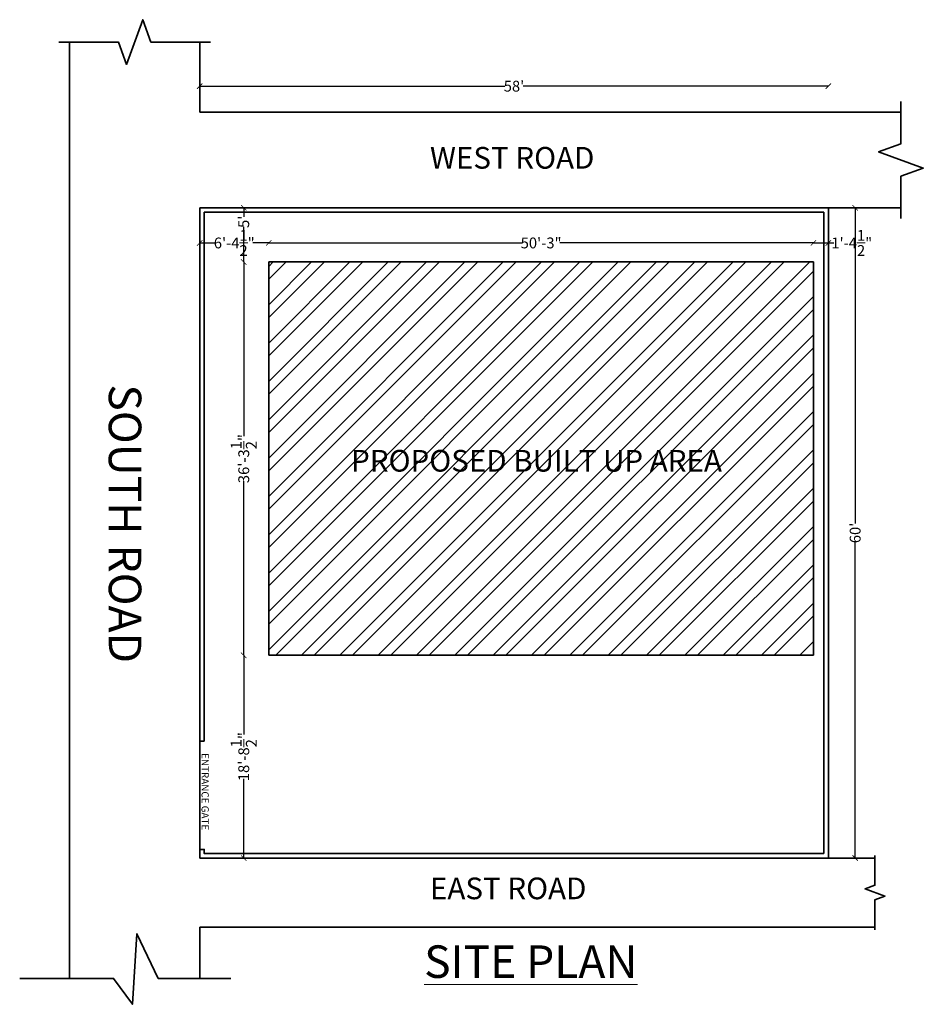
# Model space of a CAD drawing. Units: inches. Extents: x 626 to 5030, y -1681 to 1720.
# Tile 5 of 5: x 4029 to 5030, y 387 to 1477. Entities that reach past the tile are written whole.
import ezdxf

# ---------------------------------------------------------------- set-up
doc = ezdxf.new("R2010")
doc.units = ezdxf.units.IN
doc.header["$MEASUREMENT"] = 0
for name, color, linetype, lineweight in [('A-ANNO-DIMS', 2, 'Continuous', 18), ('A-ANNO-TEXT', 7, 'Continuous', 18), ('C-BLDG', 7, 'Continuous', 35), ('C-BLDG-PATT', 8, 'Continuous', 13), ('C-PROP', 1, 'Continuous', 35)]:
    doc.layers.add(name, color=color, linetype=linetype, lineweight=lineweight)
doc.styles.get("Standard").update_dxf_attribs({"font": 'arial.ttf'})
doc.dimstyles.get("Standard").update_dxf_attribs({"dimtxt": 12, "dimasz": 6, "dimexe": 0.18, "dimexo": 0.0625, "dimgap": 0.09, "dimtad": 0, "dimdec": 1, "dimzin": 0, "dimdsep": 46, "dimlunit": 4, "dimtxsty": 'Standard', "dimblk": 'ARCHTICK', "dimcen": 0.09, "dimse1": 1, "dimse2": 1, "dimclrt": 3, "dimadec": 0, "dimazin": 0, "dimtfac": 1, "dimtdec": 1, "dimtofl": 0, "dimtmove": 0, "dimatfit": 3, "dimfxl": 1, "dimtolj": 1, "dimtzin": 0, "dimarcsym": 0})

# ---------------------------------------------------------------- blocks, each defined once
blk = doc.blocks.new('_ArchTick')
at = {"color": 0, "linetype": 'ByBlock', "const_width": 0.15}
blk.add_lwpolyline([(-0.5, -0.5), (0.5, 0.5)], dxfattribs=at)
blk = doc.blocks.new('*D2')
at = {"layer": 'A-ANNO-DIMS', "color": 0, "lineweight": -2, "transparency": 16777216}
for p, q in [((4228.5, 1403.3), (4566.3, 1403.3)), ((4924.5, 1403.3), (4586.8, 1403.3))]:
    blk.add_line(p, q, dxfattribs=at)
at = {"layer": 'DEFPOINTS', "color": 0, "transparency": 16777216}
for p in [(4924.5, 1403.3), (4228.5, 1268.6), (4924.5, 1268.6)]:
    blk.add_point(p, dxfattribs=at)
at = {"layer": 'A-ANNO-DIMS', "color": 0, "lineweight": -2, "transparency": 16777216, "xscale": 6, "yscale": 6, "zscale": 6, "rotation": 180}
blk.add_blockref('_ArchTick', (4228.5, 1403.3), dxfattribs=at)
at = {"layer": 'A-ANNO-DIMS', "color": 0, "lineweight": -2, "transparency": 16777216, "xscale": 6, "yscale": 6, "zscale": 6}
blk.add_blockref('_ArchTick', (4924.5, 1403.3), dxfattribs=at)
at = {"layer": 'A-ANNO-DIMS', "color": 0, "transparency": 16777216, "insert": (4576.5, 1403.3), "char_height": 12, "attachment_point": 5}
blk.add_mtext("\\A1;58'", dxfattribs=at)
blk = doc.blocks.new('*D4')
at = {"layer": 'A-ANNO-DIMS', "color": 0, "lineweight": -2, "transparency": 16777216}
for p, q in [((4305, 1229.7), (4585.8, 1229.7)), ((4908, 1229.7), (4627.2, 1229.7))]:
    blk.add_line(p, q, dxfattribs=at)
at = {"layer": 'DEFPOINTS', "color": 0, "transparency": 16777216}
for p in [(4305, 1229.7), (4305, 1208.6), (4908, 1208.6)]:
    blk.add_point(p, dxfattribs=at)
at = {"layer": 'A-ANNO-DIMS', "color": 0, "lineweight": -2, "transparency": 16777216, "xscale": 6, "yscale": 6, "zscale": 6, "rotation": 180}
blk.add_blockref('_ArchTick', (4305, 1229.7), dxfattribs=at)
at = {"layer": 'A-ANNO-DIMS', "color": 0, "lineweight": -2, "transparency": 16777216, "xscale": 6, "yscale": 6, "zscale": 6}
blk.add_blockref('_ArchTick', (4908, 1229.7), dxfattribs=at)
at = {"layer": 'A-ANNO-DIMS', "color": 0, "transparency": 16777216, "insert": (4606.5, 1229.7), "char_height": 12, "attachment_point": 5}
blk.add_mtext('\\A1;50\'-3"', dxfattribs=at)
blk = doc.blocks.new('*D5')
at = {"layer": 'A-ANNO-DIMS', "color": 0, "lineweight": -2, "transparency": 16777216}
for p, q in [((4277.3, 1208.6), (4277.3, 1015.9)), ((4277.3, 773.1), (4277.3, 965.8))]:
    blk.add_line(p, q, dxfattribs=at)
at = {"layer": 'DEFPOINTS', "color": 0, "transparency": 16777216}
for p in [(4305, 1208.6), (4277.3, 773.1), (4305, 773.1)]:
    blk.add_point(p, dxfattribs=at)
at = {"layer": 'A-ANNO-DIMS', "color": 0, "lineweight": -2, "transparency": 16777216, "xscale": 6, "yscale": 6, "zscale": 6}
for p, rotation in [((4277.3, 1208.6), 90), ((4277.3, 773.1), 270)]:
    blk.add_blockref('_ArchTick', p, dxfattribs=dict(at, rotation=rotation))
at = {"layer": 'A-ANNO-DIMS', "color": 0, "transparency": 16777216, "insert": (4277.3, 990.9), "char_height": 12, "attachment_point": 5, "rotation": 90}
blk.add_mtext('\\A1;36\'-3{\\H1x;\\S1/2;}"', dxfattribs=at)
blk = doc.blocks.new('*D6')
at = {"layer": 'A-ANNO-DIMS', "color": 0, "lineweight": -2, "transparency": 16777216}
for p, q in [((4277.3, 773.1), (4277.3, 685.4)), ((4277.3, 548.6), (4277.3, 636.3))]:
    blk.add_line(p, q, dxfattribs=at)
at = {"layer": 'DEFPOINTS', "color": 0, "transparency": 16777216}
for p in [(4305, 773.1), (4277.3, 548.6), (4305, 548.6)]:
    blk.add_point(p, dxfattribs=at)
at = {"layer": 'A-ANNO-DIMS', "color": 0, "lineweight": -2, "transparency": 16777216, "xscale": 6, "yscale": 6, "zscale": 6}
for p, rotation in [((4277.3, 773.1), 90), ((4277.3, 548.6), 270)]:
    blk.add_blockref('_ArchTick', p, dxfattribs=dict(at, rotation=rotation))
at = {"layer": 'A-ANNO-DIMS', "color": 0, "transparency": 16777216, "insert": (4277.3, 660.9), "char_height": 12, "attachment_point": 5, "rotation": 90}
blk.add_mtext('\\A1;18\'-8{\\H1x;\\S1/2;}"', dxfattribs=at)
blk = doc.blocks.new('*D7')
at = {"layer": 'A-ANNO-DIMS', "color": 0, "lineweight": -2, "transparency": 16777216}
for p, q in [((4908, 1229.7), (4924.5, 1229.7)), ((4924.5, 1229.7), (4930.5, 1229.7))]:
    blk.add_line(p, q, dxfattribs=at)
at = {"layer": 'DEFPOINTS', "color": 0, "transparency": 16777216}
for p in [(4924.5, 1229.7), (4908, 1208.6), (4924.5, 1208.6)]:
    blk.add_point(p, dxfattribs=at)
at = {"layer": 'A-ANNO-DIMS', "color": 0, "lineweight": -2, "transparency": 16777216, "xscale": 6, "yscale": 6, "zscale": 6, "rotation": 180}
blk.add_blockref('_ArchTick', (4908, 1229.7), dxfattribs=at)
at = {"layer": 'A-ANNO-DIMS', "color": 0, "lineweight": -2, "transparency": 16777216, "xscale": 6, "yscale": 6, "zscale": 6}
blk.add_blockref('_ArchTick', (4924.5, 1229.7), dxfattribs=at)
at = {"layer": 'A-ANNO-DIMS', "color": 0, "transparency": 16777216, "insert": (4950.4, 1229.7), "char_height": 12, "attachment_point": 5}
blk.add_mtext('\\A1;1\'-4{\\H1x;\\S1/2;}"', dxfattribs=at)
blk = doc.blocks.new('*D10')
at = {"layer": 'A-ANNO-DIMS', "color": 0, "lineweight": -2, "transparency": 16777216}
for p, q in [((4228.5, 1229.7), (4246.4, 1229.7)), ((4305, 1229.7), (4287.2, 1229.7))]:
    blk.add_line(p, q, dxfattribs=at)
at = {"layer": 'DEFPOINTS', "color": 0, "transparency": 16777216}
for p in [(4228.5, 1229.7), (4228.5, 1208.6), (4305, 1208.6)]:
    blk.add_point(p, dxfattribs=at)
at = {"layer": 'A-ANNO-DIMS', "color": 0, "lineweight": -2, "transparency": 16777216, "xscale": 6, "yscale": 6, "zscale": 6, "rotation": 180}
blk.add_blockref('_ArchTick', (4228.5, 1229.7), dxfattribs=at)
at = {"layer": 'A-ANNO-DIMS', "color": 0, "lineweight": -2, "transparency": 16777216, "xscale": 6, "yscale": 6, "zscale": 6}
blk.add_blockref('_ArchTick', (4305, 1229.7), dxfattribs=at)
at = {"layer": 'A-ANNO-DIMS', "color": 0, "transparency": 16777216, "insert": (4266.8, 1229.7), "char_height": 12, "attachment_point": 5}
blk.add_mtext('\\A1;6\'-4{\\H1x;\\S1/2;}"', dxfattribs=at)
blk = doc.blocks.new('*D11')
at = {"layer": 'A-ANNO-DIMS', "color": 0, "lineweight": -2, "transparency": 16777216}
for p, q in [((4277.3, 1268.6), (4277.3, 1258.7)), ((4277.3, 1208.6), (4277.3, 1247.5))]:
    blk.add_line(p, q, dxfattribs=at)
at = {"layer": 'DEFPOINTS', "color": 0, "transparency": 16777216}
for p in [(4277.3, 1268.6), (4305, 1268.6), (4305, 1208.6)]:
    blk.add_point(p, dxfattribs=at)
at = {"layer": 'A-ANNO-DIMS', "color": 0, "lineweight": -2, "transparency": 16777216, "xscale": 6, "yscale": 6, "zscale": 6}
for p, rotation in [((4277.3, 1268.6), 90), ((4277.3, 1208.6), 270)]:
    blk.add_blockref('_ArchTick', p, dxfattribs=dict(at, rotation=rotation))
at = {"layer": 'A-ANNO-DIMS', "color": 0, "transparency": 16777216, "insert": (4277.3, 1253.1), "char_height": 12, "attachment_point": 5, "rotation": 90}
blk.add_mtext("\\A1;5'", dxfattribs=at)
blk = doc.blocks.new('*D12')
at = {"layer": 'A-ANNO-DIMS', "color": 0, "lineweight": -2, "transparency": 16777216}
for p, q in [((4954.2, 1268.6), (4954.2, 918.9)), ((4954.2, 548.6), (4954.2, 898.3))]:
    blk.add_line(p, q, dxfattribs=at)
at = {"layer": 'DEFPOINTS', "color": 0, "transparency": 16777216}
for p in [(4924.5, 1268.6), (4924.5, 548.6), (4954.2, 548.6)]:
    blk.add_point(p, dxfattribs=at)
at = {"layer": 'A-ANNO-DIMS', "color": 0, "lineweight": -2, "transparency": 16777216, "xscale": 6, "yscale": 6, "zscale": 6}
for p, rotation in [((4954.2, 1268.6), 90), ((4954.2, 548.6), 270)]:
    blk.add_blockref('_ArchTick', p, dxfattribs=dict(at, rotation=rotation))
at = {"layer": 'A-ANNO-DIMS', "color": 0, "transparency": 16777216, "insert": (4954.2, 908.6), "char_height": 12, "attachment_point": 5, "rotation": 90}
blk.add_mtext("\\A1;60'", dxfattribs=at)

msp = doc.modelspace()

# ---------------------------------------------------------------- hatches: boundary and pattern name
at = {"layer": 'C-BLDG-PATT'}
h = msp.add_hatch(dxfattribs=at)
h.set_pattern_fill('ANSI32', color=256, scale=80)
h.set_pattern_definition([(45, (3248.604, 529), (-21.2132, 21.2132), []), (45, (3262.746, 529), (-21.2132, 21.2132), [])])
h.paths.add_polyline_path([(4305.05, 1208.6), (4305.05, 773.1), (4908.05, 773.1), (4908.05, 1208.6)])
h.paths.add_polyline_path([(4387.59, 962.98), (4850.52, 962.98), (4850.52, 1012.43), (4387.59, 1012.43)], flags=24)

# ---------------------------------------------------------------- linework, layer by layer
at = {"layer": 'C-BLDG'}
for p, q in [((4908.05, 1208.6), (4305.05, 1208.6)), ((4305.05, 1208.6), (4305.05, 773.1)), ((4908.05, 773.1), (4908.05, 1208.6)), ((4305.05, 773.1), (4908.05, 773.1))]:
    msp.add_line(p, q, dxfattribs=at)
at = {"layer": 'C-PROP'}
for p, q in [((4084.55, 1452.17), (4084.55, 415.24)), ((4228.55, 1374.44), (4228.55, 1452.17)), ((5004.89, 1374.44), (4228.55, 1374.44)), ((4924.55, 1268.6), (4228.55, 1268.6)), ((4228.55, 1268.6), (4228.55, 548.6)), ((4924.55, 548.6), (4924.55, 1268.6)), ((4924.55, 1268.6), (5004.89, 1268.6)), ((4919.55, 1263.6), (4233.55, 1263.6)), ((4233.55, 1263.6), (4233.55, 678.1)), ((4919.55, 553.6), (4919.55, 1263.6)), ((4233.55, 678.1), (4228.55, 678.1)), ((4233.55, 558.1), (4233.55, 553.6)), ((4228.55, 548.6), (4924.55, 548.6)), ((4233.55, 553.6), (4919.55, 553.6)), ((4924.55, 548.6), (4976.12, 548.6)), ((4228.55, 472.21), (4976.12, 472.21)), ((4228.55, 472.21), (4228.55, 415.24))]:
    msp.add_line(p, q, dxfattribs=at)
for points in [[(4072.55, 1452.17), (4138.55, 1452.17), (4147.55, 1427.44), (4165.55, 1476.89), (4174.55, 1452.17), (4240.55, 1452.17)], [(5004.89, 1386.44), (5004.89, 1339.52), (4980.16, 1330.52), (5029.62, 1312.52), (5004.89, 1303.52), (5004.89, 1256.6)], [(4233.55, 558.1), (4233.55, 553.6), (4233.55, 558.1), (4228.55, 558.1)], [(4976.12, 469.21), (4976.12, 502.41), (4987.11, 506.41), (4965.13, 514.41), (4976.12, 518.41), (4976.12, 551.6)], [(4029.28, 415.24), (4133.3, 415.24), (4154.05, 386.66), (4159.05, 464.76), (4182.58, 415.24), (4262.92, 415.24)]]:
    msp.add_lwpolyline(points, dxfattribs=at)

# ---------------------------------------------------------------- texts
at = {"layer": 'A-ANNO-TEXT', "attachment_point": 1}
for s, width, insert, char_height in [('WEST ROAD', 299.1904, (4483.48, 1335.96), 24), ('PROPOSED BUILT UP AREA', 458.0091, (4396.18, 1000.51), 24), ('EAST ROAD', 299.1904, (4483.48, 527.01), 24), ('\\pxt25;{\\LSITE PLAN}', 352.5124, (4477.03, 451.9), 36)]:
    msp.add_mtext_dynamic_manual_height_columns(s, width=width, gutter_width=1, heights=[0], dxfattribs=dict(at, insert=insert, char_height=char_height))
at = {"layer": 'A-ANNO-TEXT', "attachment_point": 1, "rotation": 270}
for s, width, insert, char_height in [('SOUTH ROAD', 372.8618, (4163.91, 1073.1), 36), ('\\pxqc;ENTRANCE GATE', 101.9862, (4238.55, 673.1), 8)]:
    msp.add_mtext_dynamic_manual_height_columns(s, width=width, gutter_width=1, heights=[0], dxfattribs=dict(at, insert=insert, char_height=char_height))

# ---------------------------------------------------------------- dimensions: what is measured, and where the dimension line sits
at = {"layer": 'A-ANNO-DIMS'}
for base, p1, p2, picture, middle in [((4924.55, 1403.3), (4228.55, 1268.6), (4924.55, 1268.6), '*D2', (4576.55, 1403.3)), ((4228.55, 1229.7), (4305.05, 1208.6), (4228.55, 1208.6), '*D10', (4266.8, 1229.7)), ((4924.55, 1229.7), (4908.05, 1208.6), (4924.55, 1208.6), '*D7', (4950.4, 1229.7)), ((4305.05, 1229.7), (4908.05, 1208.6), (4305.05, 1208.6), '*D4', (4606.55, 1229.7))]:
    dim = msp.add_linear_dim(base=base, p1=p1, p2=p2, dimstyle='Standard', override={"dimclrd": 0, "dimclre": 0, "dimclrt": 0}, dxfattribs=at)
    dim.commit()
    dim.dimension.update_dxf_attribs({"geometry": picture, "text_midpoint": middle})
dim = msp.add_linear_dim(base=(4277.31, 1268.6), p1=(4305.05, 1208.6), p2=(4305.05, 1268.6), angle=90, dimstyle='Standard', override={"dimclrd": 0, "dimclre": 0, "dimclrt": 0}, dxfattribs=at)
dim.commit()
dim.dimension.update_dxf_attribs({"geometry": '*D11', "text_midpoint": (4277.31, 1253.07), "dimtype": 160})
for base, p1, p2, picture, middle in [((4954.16, 548.6), (4924.55, 1268.6), (4924.55, 548.6), '*D12', (4954.16, 908.6)), ((4277.31, 773.1), (4305.05, 1208.6), (4305.05, 773.1), '*D5', (4277.31, 990.85)), ((4277.31, 548.6), (4305.05, 773.1), (4305.05, 548.6), '*D6', (4277.31, 660.85))]:
    dim = msp.add_linear_dim(base=base, p1=p1, p2=p2, angle=90, dimstyle='Standard', override={"dimclrd": 0, "dimclre": 0, "dimclrt": 0}, dxfattribs=at)
    dim.commit()
    dim.dimension.update_dxf_attribs({"geometry": picture, "text_midpoint": middle})

doc.saveas('drawing.dxf')
